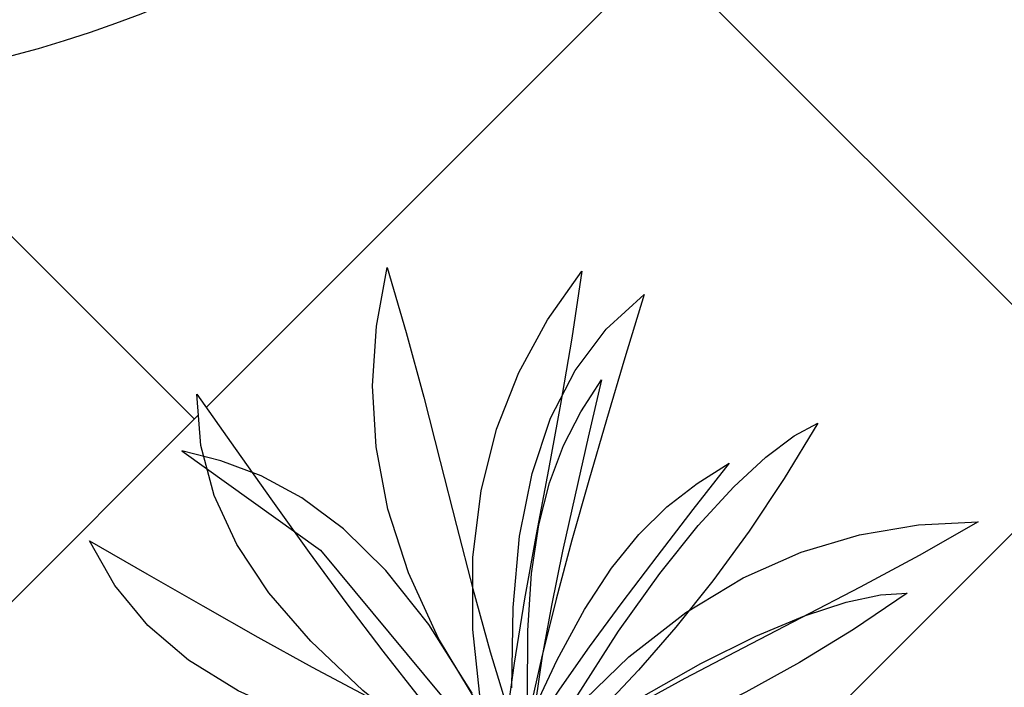
# Model space of a CAD drawing. Units: inches. Extents: x 3590 to 5167, y 65 to 1917.
# Tile 66 of 100: x 4937 to 4968, y 1702 to 1722. Entities that reach past the tile are written whole.
import ezdxf

# ---------------------------------------------------------------- set-up
doc = ezdxf.new("R2010")
doc.units = ezdxf.units.IN
for name, color, linetype, lineweight in [('A-DOOR', 3, 'Continuous', 25), ('A-FLOR-PATT', 8, 'Continuous', 13), ('L-PLNT', 94, 'Continuous', 18)]:
    doc.layers.add(name, color=color, linetype=linetype, lineweight=lineweight)
doc.layers.add('DIENHOA', color=3, linetype='Continuous')

# ---------------------------------------------------------------- blocks, each defined once
blk = doc.blocks.new('Cay03_mb')
at = {"layer": 'DIENHOA'}
for p, q in [((118.6, 555.3), (166.2, 599.1)), ((166.2, 599.1), (142.2, 519.4)), ((79.5, 503.7), (118.6, 555.3)), ((142.2, 519.4), (119, 441.7)), ((48.6, 443.6), (79.5, 503.7)), ((25.5, 374.3), (48.6, 443.6)), ((119, 441.7), (96.7, 365.6)), ((-365.2, 390.3), (-414.4, 402.8)), ((-414.4, 402.8), (-240.2, 277.8)), ((-314.9, 371.3), (-365.2, 390.3)), ((-263.5, 343.5), (-314.9, 371.3)), ((9.9, 295.3), (25.5, 374.3)), ((96.7, 365.6), (75.6, 290.6)), ((-211.2, 304.6), (-263.5, 343.5)), ((436.8, 297.2), (511, 309.6)), ((511, 309.6), (585.9, 313.5)), ((585.9, 313.5), (511.8, 271.4)), ((-158, 252.3), (-211.2, 304.6)), ((363.4, 275.4), (436.8, 297.2)), ((1.6, 205.7), (9.9, 295.3)), ((75.6, 290.6), (55.7, 216.3)), ((-240.2, 277.8), (-88.4, 94.9)), ((290.6, 243.2), (363.4, 275.4)), ((511.8, 271.4), (437.6, 231.5)), ((-104.2, 184.4), (-158, 252.3)), ((218.5, 199.8), (290.6, 243.2)), ((437.6, 231.5), (363.7, 192.9)), ((55.7, 216.3), (37.3, 142.1)), ((0.2, 104.9), (1.6, 205.7)), ((147, 144.1), (218.5, 199.8)), ((363.7, 192.9), (290.2, 154.9)), ((-49.6, 98.5), (-104.2, 184.4)), ((290.2, 154.9), (217.4, 116.6)), ((37.3, 142.1), (20.5, 67.6)), ((75.9, 75.2), (147, 144.1)), ((217.4, 116.6), (145.5, 77.3))]:
    blk.add_line(p, q, dxfattribs=at)
for points in [[(23.7, -5.4), (-41, 82.2), (-91.8, 167.1), (-129.7, 249.5), (-155.6, 329.6), (-170.2, 407.8), (-174.7, 484.2), (-169.8, 559.3), (-156.5, 633.1)], [(-156.5, 633.1), (-132.5, 551.3), (-110.5, 470), (-89.8, 389.2), (-69.6, 309), (-49, 229.4), (-27.1, 150.4), (-3.2, 72.1), (23.7, -5.4)], [(-16.4, -26.7), (-38.3, 80), (-48.9, 178.3), (-48.7, 269), (-38.5, 352.6), (-19.1, 429.7), (9, 501), (44.9, 567.1), (87.9, 628.5)], [(87.9, 628.5), (75.5, 544.2), (61.3, 461.2), (46.1, 379.1), (30.8, 297.8), (16.1, 216.9), (2.9, 136), (-8.3, 54.9), (-16.4, -26.7)], [(23.7, -5.4), (19.8, 93), (20.3, 177), (25, 248.5), (34, 309.8), (47.3, 362.7), (64.9, 409.3), (86.8, 451.7), (112.9, 491.9)], [(112.9, 491.9), (96, 419.7), (79.5, 347.4), (63.9, 276.5), (50, 208.4), (38.4, 144.8), (29.7, 86.9), (24.6, 36.3), (23.7, -5.4)], [(-395.6, 473.7), (-347.5, 405.6), (-300.6, 339.5), (-254.3, 275.1), (-208.3, 212.3), (-161.9, 150.9), (-114.8, 90.7), (-66.5, 31.6), (-16.4, -26.7)], [(-16.4, -26.7), (-108.3, 38.6), (-186.9, 101.7), (-252.4, 163.5), (-305.1, 224.4), (-345.4, 285.2), (-373.7, 346.6), (-390.4, 409.2), (-395.6, 473.7)], [(384.3, 437.5), (342.2, 367.8), (298.1, 301.7), (252.6, 239.4), (206.1, 181.1), (159.4, 127.2), (113, 78), (67.6, 33.6), (23.7, -5.4)], [(23.7, -5.4), (79.9, 91.7), (134.1, 176.2), (185.8, 248.4), (234.3, 308.7), (279, 357.3), (319.3, 394.8), (354.6, 421.4), (384.3, 437.5)], [(273.2, 387.3), (227.6, 328.8), (182.3, 270.1), (138.4, 212.3), (97.2, 156.4), (60, 103.4), (27.8, 54.6), (1.9, 10.8), (-16.4, -26.7)], [(-16.4, -26.7), (21.4, 64.2), (57, 140.3), (91.4, 203.3), (125.2, 255.1), (159.5, 297.5), (195, 332.5), (232.7, 361.8), (273.2, 387.3)], [(-530.5, 289.7), (-458.3, 248.1), (-387.9, 207.8), (-318.9, 168.7), (-250.8, 131.1), (-182.9, 94.8), (-114.9, 59.9), (-46.2, 26.5), (23.7, -5.4)], [(23.7, -5.4), (-87.2, 15.2), (-185, 39.6), (-270.3, 68.2), (-343.7, 101.4), (-405.9, 139.7), (-457.3, 183.5), (-498.7, 233.4), (-530.5, 289.7)], [(496.7, 224), (429.4, 178.4), (361.6, 136.9), (294.1, 99.5), (227.5, 66.1), (162.4, 36.7), (99.7, 11.5), (39.8, -9.7), (-16.4, -26.7)], [(-16.4, -26.7), (75.4, 37.9), (160.1, 91.8), (237.3, 135.7), (306.6, 170), (367.6, 195.4), (419.9, 212.5), (463.1, 221.9), (496.7, 224)]]:
    blk.add_lwpolyline(points, dxfattribs=at)
blk = doc.blocks.new('D1')
at = {"ltscale": 0.5}
blk.add_arc((1, 0), 34, 0, 90, dxfattribs=at)

msp = doc.modelspace()

# ---------------------------------------------------------------- hatches: boundary and pattern name
at = {"layer": 'A-FLOR-PATT', "transparency": 33554687}
h = msp.add_hatch(dxfattribs=at)
h.set_pattern_fill('AR-HBONE', color=256, scale=0.2)
h.set_pattern_definition([(45, (-588.972, 0), (0, 28.73682), [60.96, -20.32]), (135, (-574.604, 14.368), (3e-15, 28.73682), [60.96, -20.32])])
h.paths.add_polyline_path([(5071.274, 1796.999), (4933.274, 1796.999), (4933.274, 1753.999), (4962.774, 1753.999, -0.414214), (4928.774, 1719.999), (4933.274, 1718.999), (4933.274, 1334.999), (5071.274, 1334.999)])
h.paths.add_polyline_path([(4951.78, 1521.077), (4951.715, 1521.04), (4951.563, 1520.895)], flags=16)
h.paths.add_polyline_path([(4952.267, 1521.376), (4952.198, 1521.371), (4952.198, 1521.356)], flags=0)
h.paths.add_polyline_path([(4967.051, 1529.728), (4965.231, 1528.694), (4963.411, 1527.714), (4961.756, 1526.851), (4963.589, 1527.449), (4964.036, 1527.478), (4962.975, 1527.249), (4961.76, 1526.852), (4959.792, 1525.834), (4958.005, 1524.895), (4956.24, 1523.93), (4954.504, 1522.919), (4954.129, 1522.682), (4953.361, 1521.997), (4953.366, 1521.998), (4953.605, 1522.064), (4955.106, 1522.761), (4956.921, 1523.434), (4958.678, 1523.915), (4960.358, 1524.2), (4961.945, 1524.286), (4964.171, 1524.108), (4965.958, 1523.309), (4963.863, 1522.976), (4965.187, 1522.499), (4963.366, 1522.497), (4961.545, 1522.487), (4959.764, 1522.461), (4958.304, 1522.419), (4957.974, 1522.388), (4956.307, 1522.232), (4954.718, 1522.071), (4953.251, 1521.899), (4953.525, 1521.623), (4954.331, 1521.379), (4956.243, 1521.23), (4958.039, 1520.93), (4959.684, 1520.483), (4961.16, 1519.896), (4963.107, 1518.8), (4964.393, 1517.325), (4962.973, 1517.726), (4964.558, 1516.661), (4965.407, 1515.708), (4963.507, 1516.322), (4961.68, 1517.005), (4959.935, 1517.745), (4958.282, 1518.528), (4956.732, 1519.343), (4955.295, 1520.175), (4954.672, 1520.572), (4954.513, 1520.627), (4955.658, 1519.318), (4956.703, 1517.982), (4957.644, 1516.647), (4958.485, 1515.334), (4959.55, 1513.524), (4960.438, 1511.769), (4958.841, 1513.62), (4957.452, 1515.325), (4955.819, 1517.459), (4956.665, 1515.448), (4957.111, 1513.923), (4957.447, 1511.714), (4957.076, 1509.793), (4956.538, 1511.11), (4955.992, 1512.569), (4955.444, 1514.125), (4954.898, 1515.735), (4954.357, 1517.356), (4953.824, 1518.943), (4953.305, 1520.452), (4953.065, 1521.116), (4952.971, 1521.146), (4952.949, 1521.086), (4952.73, 1520.199), (4953.37, 1518.024), (4953.757, 1516.373), (4954.051, 1514.765), (4954.264, 1513.221), (4954.471, 1511.131), (4954.497, 1510.402), (4954.409, 1511.76), (4954.264, 1513.221), (4954.051, 1514.765), (4953.757, 1516.373), (4953.37, 1518.024), (4952.877, 1519.698), (4952.716, 1520.141), (4952.533, 1519.059), (4952.374, 1517.789), (4952.219, 1516.312), (4952.046, 1514.6), (4951.833, 1512.626), (4951.557, 1510.363), (4951.203, 1512.168), (4950.852, 1514.339), (4950.985, 1516.376), (4951.66, 1518.286), (4952.593, 1520.481), (4952.357, 1521.13), (4951.855, 1520.328), (4950.839, 1518.908), (4949.777, 1517.587), (4948.916, 1516.617), (4948.111, 1515.256), (4947.089, 1513.554), (4945.889, 1511.615), (4946.326, 1513.402), (4946.562, 1514.249), (4945.528, 1513.327), (4944.581, 1512.531), (4946.018, 1514.508), (4947.204, 1516.048), (4947.893, 1517.313), (4949.307, 1518.764), (4950.414, 1519.767), (4950.451, 1519.806), (4952.267, 1521.376), (4951.645, 1521.493), (4950.404, 1521.18), (4948.044, 1520.359), (4946.119, 1519.452), (4944.572, 1518.475), (4943.35, 1517.443), (4941.997, 1515.92), (4941.661, 1515.275), (4942.813, 1516.99), (4944.572, 1518.475), (4946.119, 1519.452), (4948.044, 1520.359), (4950.404, 1521.18), (4951.645, 1521.493), (4949.647, 1521.868), (4948.6, 1521.756), (4947.126, 1521.57), (4945.42, 1521.348), (4943.45, 1521.105), (4941.183, 1520.856), (4942.86, 1521.613), (4943.873, 1522.03), (4942.952, 1521.909), (4941.41, 1521.485), (4939.543, 1520.67), (4938.968, 1520.226), (4940.733, 1521.299), (4942.952, 1521.909), (4943.702, 1522.008), (4945.894, 1522.7), (4947.565, 1522.714), (4948.921, 1522.566), (4951.131, 1522.183), (4950.971, 1522.297), (4948.129, 1523.006), (4946.035, 1523.707), (4944.232, 1524.521), (4942.707, 1525.461), (4941.444, 1526.537), (4940.43, 1527.761), (4939.649, 1529.143), (4941.421, 1528.122), (4943.147, 1527.132), (4944.841, 1526.175), (4946.514, 1525.25), (4948.179, 1524.359), (4948.365, 1524.263), (4946.475, 1526.045), (4945.181, 1527.54), (4944.19, 1529.033), (4943.496, 1530.54), (4943.278, 1531.36), (4942.498, 1531.919), (4943.114, 1531.762), (4942.959, 1533.659), (4944.14, 1531.989), (4944.612, 1531.323), (4946.202, 1530.463), (4947.486, 1529.509), (4948.79, 1528.226), (4950.368, 1526.237), (4949.485, 1528.155), (4948.851, 1530.123), (4948.491, 1532.041), (4948.381, 1533.918), (4948.501, 1535.76), (4948.827, 1537.573), (4949.418, 1535.565), (4949.957, 1533.569), (4950.464, 1531.586), (4950.961, 1529.617), (4951.391, 1527.954), (4951.724, 1530.687), (4952.201, 1532.58), (4952.889, 1534.33), (4953.77, 1535.951), (4954.827, 1537.46), (4954.521, 1535.39), (4954.273, 1533.937), (4955.58, 1535.663), (4956.748, 1536.739), (4956.159, 1534.78), (4955.589, 1532.873), (4955.043, 1531.006), (4954.525, 1529.166), (4954.038, 1527.341), (4953.638, 1525.733), (4953.611, 1525.586), (4953.398, 1524.166), (4953.382, 1524.009), (4954.07, 1525.476), (4954.912, 1527.022), (4956.136, 1528.894), (4957.847, 1530.577), (4959.376, 1531.54), (4958.256, 1530.104), (4957.143, 1528.663), (4956.066, 1527.243), (4955.056, 1525.871), (4954.141, 1524.571), (4953.352, 1523.372), (4953.311, 1523.303), (4953.273, 1522.925), (4953.261, 1522.382), (4954.103, 1523.373), (4954.63, 1524.284), (4955.961, 1526.358), (4957.23, 1528.13), (4958.421, 1529.609), (4960.037, 1531.368), (4961.374, 1532.375), (4962.101, 1532.77), (4961.07, 1531.061), (4959.987, 1529.438), (4958.869, 1527.908), (4958.15, 1527.007), (4959.803, 1528.003), (4961.589, 1528.793), (4963.391, 1529.328), (4965.211, 1529.632)], flags=16)
h.paths.add_polyline_path([(4962.944, 1523.182), (4961.107, 1523.422), (4960.392, 1523.362), (4962.35, 1523.331)], flags=0)
h.paths.add_polyline_path([(5049.541, 1584.551), (5049.476, 1584.515), (5049.325, 1584.37)], flags=16)
h.paths.add_polyline_path([(5050.028, 1584.851), (5049.959, 1584.845), (5049.959, 1584.83)], flags=0)
h.paths.add_polyline_path([(5042.333, 1581.949), (5043.88, 1582.926), (5045.806, 1583.833), (5048.165, 1584.654), (5049.406, 1584.967), (5047.408, 1585.342), (5046.361, 1585.231), (5044.888, 1585.044), (5043.181, 1584.822), (5041.211, 1584.579), (5038.944, 1584.33), (5040.622, 1585.087), (5041.634, 1585.504), (5040.713, 1585.383), (5039.171, 1584.959), (5037.304, 1584.144), (5036.729, 1583.7), (5038.494, 1584.773), (5040.713, 1585.383), (5041.463, 1585.482), (5043.655, 1586.174), (5045.326, 1586.188), (5046.682, 1586.04), (5048.893, 1585.657), (5048.732, 1585.771), (5045.891, 1586.48), (5043.796, 1587.181), (5041.994, 1587.996), (5040.468, 1588.935), (5039.205, 1590.011), (5038.191, 1591.235), (5037.41, 1592.617), (5039.182, 1591.596), (5040.909, 1590.607), (5042.602, 1589.649), (5044.275, 1588.724), (5045.94, 1587.833), (5046.126, 1587.738), (5044.237, 1589.519), (5042.942, 1591.015), (5041.952, 1592.508), (5041.257, 1594.014), (5041.039, 1594.834), (5040.26, 1595.393), (5040.875, 1595.237), (5040.721, 1597.133), (5041.901, 1595.463), (5042.373, 1594.798), (5043.963, 1593.938), (5045.247, 1592.983), (5046.552, 1591.701), (5048.129, 1589.712), (5047.247, 1591.63), (5046.613, 1593.597), (5046.252, 1595.515), (5046.142, 1597.392), (5046.262, 1599.234), (5046.588, 1601.047), (5047.179, 1599.039), (5047.718, 1597.043), (5048.225, 1595.06), (5048.722, 1593.091), (5049.152, 1591.429), (5049.485, 1594.161), (5049.962, 1596.054), (5050.65, 1597.804), (5051.532, 1599.425), (5052.589, 1600.934), (5052.283, 1598.864), (5052.034, 1597.411), (5053.341, 1599.137), (5054.509, 1600.213), (5053.92, 1598.254), (5053.35, 1596.348), (5052.805, 1594.48), (5052.286, 1592.64), (5051.799, 1590.815), (5051.4, 1589.207), (5051.373, 1589.06), (5051.159, 1587.64), (5051.143, 1587.483), (5051.831, 1588.95), (5052.673, 1590.496), (5053.898, 1592.368), (5055.608, 1594.051), (5057.137, 1595.014), (5056.017, 1593.578), (5054.904, 1592.137), (5053.828, 1590.717), (5052.817, 1589.345), (5051.902, 1588.046), (5051.113, 1586.846), (5051.072, 1586.777), (5051.034, 1586.399), (5051.022, 1585.856), (5051.864, 1586.847), (5052.391, 1587.758), (5053.723, 1589.832), (5054.991, 1591.604), (5056.182, 1593.083), (5057.798, 1594.842), (5059.135, 1595.849), (5059.863, 1596.244), (5058.831, 1594.535), (5057.749, 1592.912), (5056.63, 1591.382), (5055.912, 1590.482), (5057.564, 1591.477), (5059.35, 1592.267), (5061.152, 1592.802), (5062.972, 1593.106), (5064.812, 1593.203), (5062.992, 1592.169), (5061.172, 1591.188), (5059.518, 1590.325), (5061.35, 1590.924), (5061.797, 1590.952), (5060.737, 1590.723), (5059.521, 1590.326), (5057.553, 1589.308), (5055.766, 1588.369), (5054.002, 1587.404), (5052.265, 1586.393), (5051.891, 1586.156), (5051.122, 1585.471), (5051.127, 1585.472), (5051.366, 1585.538), (5052.867, 1586.235), (5054.682, 1586.908), (5056.439, 1587.389), (5058.12, 1587.675), (5059.706, 1587.76), (5061.933, 1587.583), (5063.719, 1586.783), (5061.624, 1586.45), (5062.949, 1585.973), (5061.127, 1585.971), (5059.307, 1585.961), (5057.525, 1585.935), (5056.065, 1585.893), (5055.735, 1585.862), (5054.068, 1585.707), (5052.479, 1585.546), (5051.012, 1585.373), (5051.286, 1585.097), (5052.092, 1584.853), (5054.004, 1584.704), (5055.8, 1584.404), (5057.446, 1583.958), (5058.921, 1583.37), (5060.868, 1582.274), (5062.154, 1580.799), (5060.734, 1581.2), (5062.32, 1580.135), (5063.168, 1579.182), (5061.269, 1579.796), (5059.441, 1580.479), (5057.696, 1581.219), (5056.043, 1582.003), (5054.493, 1582.817), (5053.057, 1583.649), (5052.433, 1584.047), (5052.274, 1584.101), (5053.42, 1582.793), (5054.464, 1581.457), (5055.405, 1580.121), (5056.247, 1578.809), (5057.311, 1576.998), (5058.199, 1575.244), (5056.602, 1577.094), (5055.213, 1578.799), (5053.58, 1580.933), (5054.427, 1578.922), (5054.872, 1577.397), (5055.208, 1575.189), (5054.838, 1573.267), (5054.299, 1574.584), (5053.754, 1576.043), (5053.206, 1577.599), (5052.659, 1579.209), (5052.118, 1580.83), (5051.585, 1582.417), (5051.066, 1583.927), (5050.826, 1584.59), (5050.733, 1584.62), (5050.711, 1584.561), (5050.491, 1583.673), (5051.131, 1581.498), (5051.518, 1579.847), (5051.813, 1578.24), (5052.026, 1576.695), (5052.233, 1574.605), (5052.258, 1573.876), (5052.17, 1575.234), (5052.026, 1576.695), (5051.813, 1578.24), (5051.518, 1579.847), (5051.131, 1581.498), (5050.638, 1583.172), (5050.477, 1583.615), (5050.294, 1582.533), (5050.136, 1581.263), (5049.981, 1579.786), (5049.807, 1578.074), (5049.594, 1576.1), (5049.318, 1573.837), (5048.965, 1575.642), (5048.613, 1577.813), (5048.747, 1579.85), (5049.421, 1581.76), (5050.354, 1583.955), (5050.118, 1584.604), (5049.616, 1583.802), (5048.6, 1582.382), (5047.538, 1581.061), (5046.677, 1580.091), (5045.872, 1578.73), (5044.85, 1577.028), (5043.651, 1575.089), (5044.087, 1576.877), (5044.324, 1577.723), (5043.289, 1576.801), (5042.342, 1576.005), (5043.779, 1577.982), (5044.966, 1579.522), (5045.655, 1580.787), (5047.068, 1582.239), (5048.175, 1583.241), (5048.213, 1583.28), (5050.028, 1584.851), (5049.406, 1584.967), (5048.165, 1584.654), (5045.806, 1583.833), (5043.88, 1582.926), (5042.333, 1581.949), (5041.111, 1580.917), (5039.758, 1579.394), (5039.423, 1578.749), (5040.575, 1580.464)], flags=16)
h.paths.add_polyline_path([(4954.799, 1533.12), (4954.262, 1532.079), (4953.831, 1530.935), (4953.505, 1529.636), (4953.283, 1528.133), (4953.167, 1526.376), (4953.156, 1524.315), (4953.277, 1521.236), (4952.802, 1521.842), (4951.557, 1521.998), (4950.976, 1521.961), (4952.661, 1521.941), (4952.802, 1521.842), (4953.152, 1523.593), (4953.167, 1526.376), (4953.283, 1528.133), (4953.609, 1530.346), (4954.456, 1532.592)], flags=0)
h.paths.add_polyline_path([(5050.563, 1585.316), (5049.318, 1585.472), (5048.737, 1585.435), (5050.422, 1585.415), (5050.563, 1585.316), (5050.914, 1587.067), (5050.928, 1589.851), (5051.045, 1591.607), (5051.371, 1593.82), (5052.217, 1596.066), (5052.56, 1596.594), (5052.024, 1595.554), (5051.592, 1594.409), (5051.266, 1593.11), (5051.045, 1591.607), (5050.928, 1589.851), (5050.918, 1587.789), (5051.038, 1584.71)], flags=0)
h.paths.add_polyline_path([(5058.153, 1586.836), (5060.111, 1586.805), (5060.705, 1586.656), (5058.868, 1586.896)], flags=0)
h.paths.add_polyline_path([(5049.541, 1430.936), (5049.476, 1430.9), (5049.325, 1430.755)], flags=16)
h.paths.add_polyline_path([(5050.028, 1431.236), (5049.959, 1431.231), (5049.959, 1431.215)], flags=0)
h.paths.add_polyline_path([(5046.588, 1447.432), (5047.179, 1445.425), (5047.718, 1443.429), (5048.225, 1441.446), (5048.722, 1439.476), (5049.152, 1437.814), (5049.485, 1440.546), (5049.962, 1442.439), (5050.65, 1444.189), (5051.532, 1445.811), (5052.589, 1447.319), (5052.283, 1445.249), (5052.034, 1443.796), (5053.341, 1445.522), (5054.509, 1446.598), (5053.92, 1444.64), (5053.35, 1442.733), (5052.805, 1440.865), (5052.286, 1439.025), (5051.799, 1437.201), (5051.4, 1435.592), (5051.373, 1435.445), (5051.159, 1434.025), (5051.143, 1433.868), (5051.831, 1435.335), (5052.673, 1436.881), (5053.898, 1438.753), (5055.608, 1440.436), (5057.137, 1441.4), (5056.017, 1439.963), (5054.904, 1438.522), (5053.828, 1437.102), (5052.817, 1435.73), (5051.902, 1434.431), (5051.113, 1433.231), (5051.072, 1433.162), (5051.034, 1432.784), (5051.022, 1432.242), (5051.864, 1433.232), (5052.391, 1434.143), (5053.723, 1436.217), (5054.991, 1437.989), (5056.182, 1439.468), (5057.798, 1441.227), (5059.135, 1442.235), (5059.863, 1442.629), (5058.831, 1440.921), (5057.749, 1439.298), (5056.63, 1437.767), (5055.912, 1436.867), (5057.564, 1437.863), (5059.35, 1438.652), (5061.152, 1439.187), (5062.972, 1439.491), (5064.812, 1439.588), (5062.992, 1438.554), (5061.172, 1437.573), (5059.518, 1436.71), (5061.35, 1437.309), (5061.797, 1437.337), (5060.737, 1437.108), (5059.521, 1436.711), (5057.553, 1435.693), (5055.766, 1434.754), (5054.002, 1433.789), (5052.265, 1432.778), (5051.891, 1432.541), (5051.122, 1431.856), (5051.127, 1431.857), (5051.366, 1431.923), (5052.867, 1432.62), (5054.682, 1433.293), (5056.439, 1433.775), (5058.12, 1434.06), (5059.706, 1434.145), (5061.933, 1433.968), (5063.719, 1433.168), (5061.624, 1432.835), (5062.949, 1432.358), (5061.127, 1432.357), (5059.307, 1432.346), (5057.525, 1432.32), (5056.065, 1432.278), (5055.735, 1432.248), (5054.068, 1432.092), (5052.479, 1431.931), (5051.012, 1431.759), (5051.286, 1431.482), (5052.092, 1431.238), (5054.004, 1431.089), (5055.8, 1430.789), (5057.446, 1430.343), (5058.921, 1429.755), (5060.868, 1428.66), (5062.154, 1427.185), (5060.734, 1427.585), (5062.32, 1426.52), (5063.168, 1425.567), (5061.269, 1426.181), (5059.441, 1426.865), (5057.696, 1427.604), (5056.043, 1428.388), (5054.493, 1429.202), (5053.057, 1430.034), (5052.433, 1430.432), (5052.274, 1430.487), (5053.42, 1429.178), (5054.464, 1427.842), (5055.405, 1426.506), (5056.247, 1425.194), (5057.311, 1423.383), (5058.199, 1421.629), (5056.602, 1423.479), (5055.213, 1425.184), (5053.58, 1427.318), (5054.427, 1425.307), (5054.872, 1423.782), (5055.208, 1421.574), (5054.838, 1419.652), (5054.299, 1420.97), (5053.754, 1422.428), (5053.206, 1423.984), (5052.659, 1425.595), (5052.118, 1427.215), (5051.585, 1428.802), (5051.066, 1430.312), (5050.826, 1430.975), (5050.733, 1431.005), (5050.711, 1430.946), (5050.491, 1430.058), (5051.131, 1427.883), (5051.518, 1426.232), (5051.813, 1424.625), (5052.026, 1423.081), (5052.233, 1420.991), (5052.258, 1420.261), (5052.17, 1421.619), (5052.026, 1423.081), (5051.813, 1424.625), (5051.518, 1426.232), (5051.131, 1427.883), (5050.638, 1429.558), (5050.477, 1430.001), (5050.294, 1428.918), (5050.136, 1427.648), (5049.981, 1426.171), (5049.807, 1424.459), (5049.594, 1422.485), (5049.318, 1420.222), (5048.965, 1422.028), (5048.613, 1424.199), (5048.747, 1426.235), (5049.421, 1428.146), (5050.354, 1430.34), (5050.118, 1430.989), (5049.616, 1430.187), (5048.6, 1428.768), (5047.538, 1427.446), (5046.677, 1426.477), (5045.872, 1425.116), (5044.85, 1423.413), (5043.651, 1421.474), (5044.087, 1423.262), (5044.324, 1424.109), (5043.289, 1423.186), (5042.342, 1422.391), (5043.779, 1424.368), (5044.966, 1425.907), (5045.655, 1427.173), (5047.068, 1428.624), (5048.175, 1429.627), (5048.213, 1429.666), (5050.028, 1431.236), (5049.406, 1431.353), (5048.165, 1431.039), (5045.806, 1430.218), (5043.88, 1429.311), (5042.333, 1428.334), (5041.111, 1427.302), (5039.758, 1425.779), (5039.423, 1425.134), (5040.575, 1426.849), (5042.333, 1428.334), (5043.88, 1429.311), (5045.806, 1430.218), (5048.165, 1431.039), (5049.406, 1431.353), (5047.408, 1431.727), (5046.361, 1431.616), (5044.888, 1431.429), (5043.181, 1431.207), (5041.211, 1430.964), (5038.944, 1430.715), (5040.622, 1431.472), (5041.634, 1431.89), (5040.713, 1431.769), (5039.171, 1431.345), (5037.304, 1430.53), (5036.729, 1430.085), (5038.494, 1431.158), (5040.713, 1431.769), (5041.463, 1431.867), (5043.655, 1432.559), (5045.326, 1432.573), (5046.682, 1432.425), (5048.893, 1432.042), (5048.732, 1432.156), (5045.891, 1432.865), (5043.796, 1433.566), (5041.994, 1434.381), (5040.468, 1435.321), (5039.205, 1436.396), (5038.191, 1437.62), (5037.41, 1439.002), (5039.182, 1437.982), (5040.909, 1436.992), (5042.602, 1436.034), (5044.275, 1435.109), (5045.94, 1434.218), (5046.126, 1434.123), (5044.237, 1435.904), (5042.942, 1437.4), (5041.952, 1438.893), (5041.257, 1440.399), (5041.039, 1441.219), (5040.26, 1441.778), (5040.875, 1441.622), (5040.721, 1443.518), (5041.901, 1441.848), (5042.373, 1441.183), (5043.963, 1440.323), (5045.247, 1439.369), (5046.552, 1438.086), (5048.129, 1436.097), (5047.247, 1438.015), (5046.613, 1439.982), (5046.252, 1441.901), (5046.142, 1443.778), (5046.262, 1445.619)], flags=16)
h.paths.add_polyline_path([(5052.382, 1444.255), (5051.623, 1442.78), (5052.024, 1441.939), (5052.56, 1442.98)], flags=0)
h.paths.add_polyline_path([(5050.563, 1431.701), (5049.318, 1431.857), (5048.737, 1431.821), (5050.422, 1431.8)], flags=0)
h.paths.add_polyline_path([(5058.153, 1433.221), (5060.111, 1433.19), (5060.705, 1433.041), (5058.868, 1433.281)], flags=0)
h.paths.add_polyline_path([(5049.541, 1352.285), (5049.476, 1352.249), (5049.325, 1352.104)], flags=16)
h.paths.add_polyline_path([(5050.028, 1352.585), (5049.959, 1352.58), (5049.959, 1352.564)], flags=0)
h.paths.add_polyline_path([(5046.588, 1368.781), (5047.179, 1366.774), (5047.718, 1364.778), (5048.225, 1362.795), (5048.722, 1360.825), (5049.152, 1359.163), (5049.485, 1361.896), (5049.962, 1363.789), (5050.65, 1365.538), (5051.532, 1367.16), (5052.589, 1368.669), (5052.283, 1366.598), (5052.034, 1365.145), (5053.341, 1366.871), (5054.509, 1367.947), (5053.92, 1365.989), (5053.35, 1364.082), (5052.805, 1362.214), (5052.286, 1360.374), (5051.799, 1358.55), (5051.4, 1356.942), (5051.373, 1356.794), (5051.159, 1355.374), (5051.143, 1355.218), (5051.831, 1356.684), (5052.673, 1358.23), (5053.898, 1360.102), (5055.608, 1361.786), (5057.137, 1362.749), (5056.017, 1361.313), (5054.904, 1359.872), (5053.828, 1358.452), (5052.817, 1357.079), (5051.902, 1355.78), (5051.113, 1354.581), (5051.072, 1354.512), (5051.034, 1354.133), (5051.022, 1353.591), (5051.864, 1354.581), (5052.391, 1355.492), (5053.723, 1357.566), (5054.991, 1359.338), (5056.182, 1360.817), (5057.798, 1362.577), (5059.135, 1363.584), (5059.863, 1363.979), (5058.831, 1362.27), (5057.749, 1360.647), (5056.63, 1359.117), (5055.912, 1358.216), (5057.564, 1359.212), (5059.35, 1360.001), (5061.152, 1360.536), (5062.972, 1360.841), (5064.812, 1360.937), (5062.992, 1359.903), (5061.172, 1358.923), (5059.518, 1358.059), (5061.35, 1358.658), (5061.797, 1358.687), (5060.737, 1358.458), (5059.521, 1358.061), (5057.553, 1357.043), (5055.766, 1356.103), (5054.002, 1355.138), (5052.265, 1354.127), (5051.891, 1353.89), (5051.122, 1353.206), (5051.127, 1353.206), (5051.366, 1353.272), (5052.867, 1353.969), (5054.682, 1354.643), (5056.439, 1355.124), (5058.12, 1355.409), (5059.706, 1355.495), (5061.933, 1355.317), (5063.719, 1354.518), (5061.624, 1354.184), (5062.949, 1353.708), (5061.127, 1353.706), (5059.307, 1353.695), (5057.525, 1353.669), (5056.065, 1353.627), (5055.735, 1353.597), (5054.068, 1353.441), (5052.479, 1353.28), (5051.012, 1353.108), (5051.286, 1352.831), (5052.092, 1352.587), (5054.004, 1352.439), (5055.8, 1352.138), (5057.446, 1351.692), (5058.921, 1351.104), (5060.868, 1350.009), (5062.154, 1348.534), (5060.734, 1348.935), (5062.32, 1347.869), (5063.168, 1346.916), (5061.269, 1347.53), (5059.441, 1348.214), (5057.696, 1348.954), (5056.043, 1349.737), (5054.493, 1350.551), (5053.057, 1351.383), (5052.433, 1351.781), (5052.274, 1351.836), (5053.42, 1350.527), (5054.464, 1349.191), (5055.405, 1347.855), (5056.247, 1346.543), (5057.311, 1344.733), (5058.199, 1342.978), (5056.602, 1344.828), (5055.213, 1346.534), (5053.58, 1348.667), (5054.427, 1346.656), (5054.872, 1345.132), (5055.208, 1342.923), (5054.838, 1341.002), (5054.299, 1342.319), (5053.754, 1343.778), (5053.206, 1345.334), (5052.659, 1346.944), (5052.118, 1348.564), (5051.585, 1350.151), (5051.066, 1351.661), (5050.826, 1352.324), (5050.733, 1352.355), (5050.711, 1352.295), (5050.491, 1351.408), (5051.131, 1349.232), (5051.518, 1347.581), (5051.813, 1345.974), (5052.026, 1344.43), (5052.233, 1342.34), (5052.258, 1341.61), (5052.17, 1342.969), (5052.026, 1344.43), (5051.813, 1345.974), (5051.518, 1347.581), (5051.131, 1349.232), (5050.638, 1350.907), (5050.477, 1351.35), (5050.294, 1350.267), (5050.136, 1348.997), (5049.981, 1347.52), (5049.807, 1345.809), (5049.594, 1343.835), (5049.318, 1341.571), (5048.965, 1343.377), (5048.613, 1345.548), (5048.747, 1347.585), (5049.421, 1349.495), (5050.354, 1351.689), (5050.118, 1352.339), (5049.616, 1351.536), (5048.6, 1350.117), (5047.538, 1348.795), (5046.677, 1347.826), (5045.872, 1346.465), (5044.85, 1344.763), (5043.651, 1342.824), (5044.087, 1344.611), (5044.324, 1345.458), (5043.289, 1344.535), (5042.342, 1343.74), (5043.779, 1345.717), (5044.966, 1347.256), (5045.655, 1348.522), (5047.068, 1349.973), (5048.175, 1350.976), (5048.213, 1351.015), (5050.028, 1352.585), (5049.406, 1352.702), (5048.165, 1352.388), (5045.806, 1351.567), (5043.88, 1350.661), (5042.333, 1349.683), (5041.111, 1348.651), (5039.758, 1347.128), (5039.423, 1346.483), (5040.575, 1348.198), (5042.333, 1349.683), (5043.88, 1350.661), (5045.806, 1351.567), (5048.165, 1352.388), (5049.406, 1352.702), (5047.408, 1353.076), (5046.361, 1352.965), (5044.888, 1352.779), (5043.181, 1352.556), (5041.211, 1352.313), (5038.944, 1352.065), (5040.622, 1352.821), (5041.634, 1353.239), (5040.713, 1353.118), (5039.171, 1352.694), (5037.304, 1351.879), (5036.729, 1351.434), (5038.494, 1352.508), (5040.713, 1353.118), (5041.463, 1353.216), (5043.655, 1353.909), (5045.326, 1353.923), (5046.682, 1353.774), (5048.893, 1353.391), (5048.732, 1353.506), (5045.891, 1354.214), (5043.796, 1354.915), (5041.994, 1355.73), (5040.468, 1356.67), (5039.205, 1357.746), (5038.191, 1358.969), (5037.41, 1360.352), (5039.182, 1359.331), (5040.909, 1358.341), (5042.602, 1357.383), (5044.275, 1356.458), (5045.94, 1355.567), (5046.126, 1355.472), (5044.237, 1357.253), (5042.942, 1358.749), (5041.952, 1360.242), (5041.257, 1361.748), (5041.039, 1362.568), (5040.26, 1363.128), (5040.875, 1362.971), (5040.721, 1364.867), (5041.901, 1363.197), (5042.373, 1362.532), (5043.963, 1361.672), (5045.247, 1360.718), (5046.552, 1359.435), (5048.129, 1357.446), (5047.247, 1359.364), (5046.613, 1361.331), (5046.252, 1363.25), (5046.142, 1365.127), (5046.262, 1366.969)], flags=16)
h.paths.add_polyline_path([(5052.382, 1365.604), (5051.623, 1364.129), (5052.024, 1363.288), (5052.56, 1364.329)], flags=0)
h.paths.add_polyline_path([(4951.78, 1698.041), (4951.715, 1698.005), (4951.563, 1697.859)], flags=16)
h.paths.add_polyline_path([(4952.267, 1698.341), (4952.198, 1698.335), (4952.198, 1698.32)], flags=0)
h.paths.add_polyline_path([(4957.076, 1686.757), (4956.538, 1688.074), (4955.992, 1689.533), (4955.444, 1691.089), (4954.898, 1692.699), (4954.357, 1694.32), (4953.824, 1695.907), (4953.305, 1697.417), (4953.065, 1698.08), (4952.971, 1698.11), (4952.949, 1698.051), (4952.73, 1697.163), (4953.37, 1694.988), (4953.757, 1693.337), (4954.051, 1691.729), (4954.264, 1690.185), (4954.471, 1688.095), (4954.497, 1687.366), (4954.409, 1688.724), (4954.264, 1690.185), (4954.051, 1691.729), (4953.757, 1693.337), (4953.37, 1694.988), (4952.877, 1696.662), (4952.716, 1697.105), (4952.533, 1696.023), (4952.374, 1694.753), (4952.219, 1693.276), (4952.046, 1691.564), (4951.833, 1689.59), (4951.557, 1687.327), (4951.203, 1689.132), (4950.852, 1691.303), (4950.985, 1693.34), (4951.66, 1695.25), (4952.593, 1697.445), (4952.357, 1698.094), (4951.855, 1697.292), (4950.839, 1695.872), (4949.777, 1694.551), (4948.916, 1693.581), (4948.111, 1692.22), (4947.089, 1690.518), (4945.889, 1688.579), (4946.326, 1690.366), (4946.562, 1691.213), (4945.528, 1690.291), (4944.581, 1689.495), (4946.018, 1691.472), (4947.204, 1693.012), (4947.893, 1694.277), (4949.307, 1695.729), (4950.414, 1696.731), (4950.451, 1696.77), (4952.267, 1698.341), (4951.645, 1698.457), (4950.404, 1698.144), (4948.044, 1697.323), (4946.119, 1696.416), (4944.572, 1695.439), (4943.35, 1694.407), (4941.997, 1692.884), (4941.661, 1692.239), (4942.813, 1693.954), (4944.572, 1695.439), (4946.119, 1696.416), (4948.044, 1697.323), (4950.404, 1698.144), (4951.645, 1698.457), (4949.647, 1698.832), (4948.6, 1698.72), (4947.126, 1698.534), (4945.42, 1698.312), (4943.45, 1698.069), (4941.183, 1697.82), (4942.86, 1698.577), (4943.873, 1698.994), (4942.952, 1698.873), (4941.41, 1698.449), (4939.543, 1697.634), (4938.968, 1697.19), (4940.733, 1698.263), (4942.952, 1698.873), (4943.702, 1698.972), (4945.894, 1699.664), (4947.565, 1699.678), (4948.921, 1699.53), (4951.131, 1699.147), (4950.971, 1699.261), (4948.129, 1699.97), (4946.035, 1700.671), (4944.232, 1701.486), (4942.707, 1702.425), (4941.444, 1703.501), (4940.43, 1704.725), (4939.649, 1706.107), (4941.421, 1705.086), (4943.147, 1704.097), (4944.841, 1703.139), (4946.514, 1702.214), (4948.179, 1701.323), (4948.365, 1701.227), (4946.475, 1703.009), (4945.181, 1704.505), (4944.19, 1705.997), (4943.496, 1707.504), (4943.278, 1708.324), (4942.498, 1708.883), (4943.114, 1708.727), (4942.959, 1710.623), (4944.14, 1708.953), (4944.612, 1708.287), (4946.202, 1707.428), (4947.486, 1706.473), (4948.79, 1705.191), (4950.368, 1703.202), (4949.485, 1705.12), (4948.851, 1707.087), (4948.491, 1709.005), (4948.381, 1710.882), (4948.501, 1712.724), (4948.827, 1714.537), (4949.418, 1712.529), (4949.957, 1710.533), (4950.464, 1708.55), (4950.961, 1706.581), (4951.391, 1704.919), (4951.724, 1707.651), (4952.201, 1709.544), (4952.889, 1711.294), (4953.77, 1712.915), (4954.827, 1714.424), (4954.521, 1712.354), (4954.273, 1710.901), (4955.58, 1712.627), (4956.748, 1713.703), (4956.159, 1711.744), (4955.589, 1709.837), (4955.043, 1707.97), (4954.525, 1706.13), (4954.038, 1704.305), (4953.638, 1702.697), (4953.611, 1702.55), (4953.398, 1701.13), (4953.382, 1700.973), (4954.07, 1702.44), (4954.912, 1703.986), (4956.136, 1705.858), (4957.847, 1707.541), (4959.376, 1708.504), (4958.256, 1707.068), (4957.143, 1705.627), (4956.066, 1704.207), (4955.056, 1702.835), (4954.141, 1701.536), (4953.352, 1700.336), (4953.311, 1700.267), (4953.273, 1699.889), (4953.261, 1699.346), (4954.103, 1700.337), (4954.63, 1701.248), (4955.961, 1703.322), (4957.23, 1705.094), (4958.421, 1706.573), (4960.037, 1708.332), (4961.374, 1709.339), (4962.101, 1709.734), (4961.07, 1708.025), (4959.987, 1706.402), (4958.869, 1704.872), (4958.15, 1703.972), (4959.803, 1704.967), (4961.589, 1705.757), (4963.391, 1706.292), (4965.211, 1706.596), (4967.051, 1706.692), (4965.231, 1705.659), (4963.411, 1704.678), (4961.756, 1703.815), (4963.589, 1704.413), (4964.036, 1704.442), (4962.975, 1704.213), (4961.76, 1703.816), (4959.792, 1702.798), (4958.005, 1701.859), (4956.24, 1700.894), (4954.504, 1699.883), (4954.129, 1699.646), (4953.361, 1698.961), (4953.366, 1698.962), (4953.605, 1699.028), (4955.106, 1699.725), (4956.921, 1700.398), (4958.678, 1700.879), (4960.358, 1701.164), (4961.945, 1701.25), (4964.171, 1701.073), (4965.958, 1700.273), (4963.863, 1699.94), (4965.187, 1699.463), (4963.366, 1699.461), (4961.545, 1699.451), (4959.764, 1699.425), (4958.304, 1699.383), (4957.974, 1699.352), (4956.307, 1699.197), (4954.718, 1699.036), (4953.251, 1698.863), (4953.525, 1698.587), (4954.331, 1698.343), (4956.243, 1698.194), (4958.039, 1697.894), (4959.684, 1697.447), (4961.16, 1696.86), (4963.107, 1695.764), (4964.393, 1694.289), (4962.973, 1694.69), (4964.558, 1693.625), (4965.407, 1692.672), (4963.507, 1693.286), (4961.68, 1693.969), (4959.935, 1694.709), (4958.282, 1695.492), (4956.732, 1696.307), (4955.295, 1697.139), (4954.672, 1697.536), (4954.513, 1697.591), (4955.658, 1696.282), (4956.703, 1694.946), (4957.644, 1693.611), (4958.485, 1692.298), (4959.55, 1690.488), (4960.438, 1688.733), (4958.841, 1690.584), (4957.452, 1692.289), (4955.819, 1694.423), (4956.665, 1692.412), (4957.111, 1690.887), (4957.447, 1688.678)], flags=16)
h.paths.add_polyline_path([(5050.563, 1353.05), (5049.318, 1353.207), (5048.737, 1353.17), (5050.422, 1353.15)], flags=0)
h.paths.add_polyline_path([(4951.78, 1351.486), (4951.715, 1351.45), (4951.563, 1351.305)], flags=16)
h.paths.add_polyline_path([(4952.267, 1351.786), (4952.198, 1351.78), (4952.198, 1351.765)], flags=0)
h.paths.add_polyline_path([(4954.827, 1367.869), (4954.521, 1365.799), (4954.273, 1364.346), (4955.58, 1366.072), (4956.748, 1367.148), (4956.159, 1365.19), (4955.589, 1363.283), (4955.043, 1361.415), (4954.525, 1359.575), (4954.038, 1357.751), (4953.638, 1356.142), (4953.611, 1355.995), (4953.398, 1354.575), (4953.382, 1354.418), (4954.07, 1355.885), (4954.912, 1357.431), (4956.136, 1359.303), (4957.847, 1360.986), (4959.376, 1361.95), (4958.256, 1360.513), (4957.143, 1359.072), (4956.066, 1357.652), (4955.056, 1356.28), (4954.141, 1354.981), (4953.352, 1353.781), (4953.311, 1353.712), (4953.273, 1353.334), (4953.261, 1352.792), (4954.103, 1353.782), (4954.63, 1354.693), (4955.961, 1356.767), (4957.23, 1358.539), (4958.421, 1360.018), (4960.037, 1361.777), (4961.374, 1362.785), (4962.101, 1363.179), (4961.07, 1361.471), (4959.987, 1359.848), (4958.869, 1358.317), (4958.15, 1357.417), (4959.803, 1358.413), (4961.589, 1359.202), (4963.391, 1359.737), (4965.211, 1360.041), (4967.051, 1360.138), (4965.231, 1359.104), (4963.411, 1358.123), (4961.756, 1357.26), (4963.589, 1357.859), (4964.036, 1357.887), (4962.975, 1357.658), (4961.76, 1357.261), (4959.792, 1356.243), (4958.005, 1355.304), (4956.24, 1354.339), (4954.504, 1353.328), (4954.129, 1353.091), (4953.361, 1352.406), (4953.366, 1352.407), (4953.605, 1352.473), (4955.106, 1353.17), (4956.921, 1353.843), (4958.678, 1354.325), (4960.358, 1354.61), (4961.945, 1354.695), (4964.171, 1354.518), (4965.958, 1353.718), (4963.863, 1353.385), (4965.187, 1352.908), (4963.366, 1352.907), (4961.545, 1352.896), (4959.764, 1352.87), (4958.304, 1352.828), (4957.974, 1352.798), (4956.307, 1352.642), (4954.718, 1352.481), (4953.251, 1352.309), (4953.525, 1352.032), (4954.331, 1351.788), (4956.243, 1351.639), (4958.039, 1351.339), (4959.684, 1350.893), (4961.16, 1350.305), (4963.107, 1349.21), (4964.393, 1347.735), (4962.973, 1348.135), (4964.558, 1347.07), (4965.407, 1346.117), (4963.507, 1346.731), (4961.68, 1347.414), (4959.935, 1348.154), (4958.282, 1348.938), (4956.732, 1349.752), (4955.295, 1350.584), (4954.672, 1350.982), (4954.513, 1351.036), (4955.658, 1349.728), (4956.703, 1348.392), (4957.644, 1347.056), (4958.485, 1345.744), (4959.55, 1343.933), (4960.438, 1342.179), (4958.841, 1344.029), (4957.452, 1345.734), (4955.819, 1347.868), (4956.665, 1345.857), (4957.111, 1344.332), (4957.447, 1342.124), (4957.076, 1340.202), (4956.538, 1341.52), (4955.992, 1342.978), (4955.444, 1344.534), (4954.898, 1346.145), (4954.357, 1347.765), (4953.824, 1349.352), (4953.305, 1350.862), (4953.065, 1351.525), (4952.971, 1351.555), (4952.949, 1351.496), (4952.73, 1350.608), (4953.37, 1348.433), (4953.757, 1346.782), (4954.051, 1345.175), (4954.264, 1343.631), (4954.471, 1341.541), (4954.497, 1340.811), (4954.409, 1342.169), (4954.264, 1343.631), (4954.051, 1345.175), (4953.757, 1346.782), (4953.37, 1348.433), (4952.877, 1350.108), (4952.716, 1350.551), (4952.533, 1349.468), (4952.374, 1348.198), (4952.219, 1346.721), (4952.046, 1345.009), (4951.833, 1343.035), (4951.557, 1340.772), (4951.203, 1342.578), (4950.852, 1344.749), (4950.985, 1346.785), (4951.66, 1348.696), (4952.593, 1350.89), (4952.357, 1351.539), (4951.855, 1350.737), (4950.839, 1349.318), (4949.777, 1347.996), (4948.916, 1347.027), (4948.111, 1345.665), (4947.089, 1343.963), (4945.889, 1342.024), (4946.326, 1343.812), (4946.562, 1344.659), (4945.528, 1343.736), (4944.581, 1342.941), (4946.018, 1344.918), (4947.204, 1346.457), (4947.893, 1347.723), (4949.307, 1349.174), (4950.414, 1350.177), (4950.451, 1350.216), (4952.267, 1351.786), (4951.645, 1351.903), (4950.404, 1351.589), (4948.044, 1350.768), (4946.119, 1349.861), (4944.572, 1348.884), (4943.35, 1347.852), (4941.997, 1346.329), (4941.661, 1345.684), (4942.813, 1347.399), (4944.572, 1348.884), (4946.119, 1349.861), (4948.044, 1350.768), (4950.404, 1351.589), (4951.645, 1351.903), (4949.647, 1352.277), (4948.6, 1352.166), (4947.126, 1351.979), (4945.42, 1351.757), (4943.45, 1351.514), (4941.183, 1351.265), (4942.86, 1352.022), (4943.873, 1352.44), (4942.952, 1352.319), (4941.41, 1351.895), (4939.543, 1351.08), (4938.968, 1350.635), (4940.733, 1351.708), (4942.952, 1352.319), (4943.702, 1352.417), (4945.894, 1353.109), (4947.565, 1353.123), (4948.921, 1352.975), (4951.131, 1352.592), (4950.971, 1352.706), (4948.129, 1353.415), (4946.035, 1354.116), (4944.232, 1354.931), (4942.707, 1355.871), (4941.444, 1356.946), (4940.43, 1358.17), (4939.649, 1359.552), (4941.421, 1358.532), (4943.147, 1357.542), (4944.841, 1356.584), (4946.514, 1355.659), (4948.179, 1354.768), (4948.365, 1354.673), (4946.475, 1356.454), (4945.181, 1357.95), (4944.19, 1359.443), (4943.496, 1360.949), (4943.278, 1361.769), (4942.498, 1362.328), (4943.114, 1362.172), (4942.959, 1364.068), (4944.14, 1362.398), (4944.612, 1361.733), (4946.202, 1360.873), (4947.486, 1359.919), (4948.79, 1358.636), (4950.368, 1356.647), (4949.485, 1358.565), (4948.851, 1360.532), (4948.491, 1362.451), (4948.381, 1364.328), (4948.501, 1366.169), (4948.827, 1367.982), (4949.418, 1365.975), (4949.957, 1363.979), (4950.464, 1361.995), (4950.961, 1360.026), (4951.391, 1358.364), (4951.724, 1361.096), (4952.201, 1362.989), (4952.889, 1364.739), (4953.77, 1366.361)], flags=16)
h.paths.add_polyline_path([(4954.799, 1363.53), (4954.262, 1362.489), (4953.831, 1361.344), (4953.505, 1360.045), (4953.283, 1358.543), (4953.167, 1356.786), (4953.156, 1354.724), (4953.277, 1351.646), (4952.802, 1352.251), (4951.557, 1352.407), (4950.976, 1352.371), (4952.661, 1352.35), (4952.802, 1352.251), (4953.152, 1354.002), (4953.167, 1356.786), (4953.283, 1358.543), (4953.609, 1360.755), (4954.456, 1363.001)], flags=0)
h.paths.add_polyline_path([(4952.802, 1698.806), (4951.557, 1698.962), (4950.976, 1698.925), (4952.661, 1698.905), (4952.802, 1698.806), (4953.152, 1700.557), (4953.167, 1703.34), (4953.283, 1705.097), (4953.609, 1707.31), (4954.456, 1709.556), (4954.799, 1710.084), (4954.262, 1709.043), (4953.831, 1707.899), (4953.505, 1706.6), (4953.283, 1705.097), (4953.167, 1703.34), (4953.156, 1701.279), (4953.277, 1698.2)], flags=0)
h.paths.add_polyline_path([(4962.944, 1700.146), (4961.107, 1700.386), (4960.392, 1700.326), (4962.35, 1700.295)], flags=0)
h.paths.add_polyline_path([(5058.153, 1354.57), (5060.111, 1354.539), (5060.705, 1354.391), (5058.868, 1354.631)], flags=0)
h.paths.add_polyline_path([(4962.944, 1353.591), (4961.107, 1353.831), (4960.392, 1353.771), (4962.35, 1353.74)], flags=0)
h.paths.add_polyline_path([(5049.541, 1778.72), (5049.476, 1778.684), (5049.325, 1778.539)], flags=16)
h.paths.add_polyline_path([(5050.028, 1779.02), (5049.959, 1779.014), (5049.959, 1778.999)], flags=0)
h.paths.add_polyline_path([(5052.258, 1768.045), (5052.17, 1769.403), (5052.026, 1770.864), (5051.813, 1772.409), (5051.518, 1774.016), (5051.131, 1775.667), (5050.638, 1777.341), (5050.477, 1777.784), (5050.294, 1776.702), (5050.136, 1775.432), (5049.981, 1773.955), (5049.807, 1772.243), (5049.594, 1770.269), (5049.318, 1768.006), (5048.965, 1769.811), (5048.613, 1771.982), (5048.747, 1774.019), (5049.421, 1775.929), (5050.354, 1778.124), (5050.118, 1778.773), (5049.616, 1777.971), (5048.6, 1776.551), (5047.538, 1775.23), (5046.677, 1774.26), (5045.872, 1772.899), (5044.85, 1771.197), (5043.651, 1769.258), (5044.087, 1771.046), (5044.324, 1771.892), (5043.289, 1770.97), (5042.342, 1770.174), (5043.779, 1772.151), (5044.966, 1773.691), (5045.655, 1774.956), (5047.068, 1776.408), (5048.175, 1777.41), (5048.213, 1777.449), (5050.028, 1779.02), (5049.406, 1779.136), (5048.165, 1778.823), (5045.806, 1778.002), (5043.88, 1777.095), (5042.333, 1776.118), (5041.111, 1775.086), (5039.758, 1773.563), (5039.423, 1772.918), (5040.575, 1774.633), (5042.333, 1776.118), (5043.88, 1777.095), (5045.806, 1778.002), (5048.165, 1778.823), (5049.406, 1779.136), (5047.408, 1779.511), (5046.361, 1779.4), (5044.888, 1779.213), (5043.181, 1778.991), (5041.211, 1778.748), (5038.944, 1778.499), (5040.622, 1779.256), (5041.634, 1779.673), (5040.713, 1779.552), (5039.171, 1779.128), (5037.304, 1778.313), (5036.729, 1777.869), (5038.494, 1778.942), (5040.713, 1779.552), (5041.463, 1779.651), (5043.655, 1780.343), (5045.326, 1780.357), (5046.682, 1780.209), (5048.893, 1779.826), (5048.732, 1779.94), (5045.891, 1780.649), (5043.796, 1781.35), (5041.994, 1782.165), (5040.468, 1783.104), (5039.205, 1784.18), (5038.191, 1785.404), (5037.41, 1786.786), (5039.182, 1785.765), (5040.909, 1784.776), (5042.602, 1783.818), (5044.275, 1782.893), (5045.94, 1782.002), (5046.126, 1781.907), (5044.237, 1783.688), (5042.942, 1785.184), (5041.952, 1786.677), (5041.257, 1788.183), (5041.039, 1789.003), (5040.26, 1789.562), (5040.875, 1789.406), (5040.721, 1791.302), (5041.901, 1789.632), (5042.373, 1788.967), (5043.963, 1788.107), (5045.247, 1787.152), (5046.552, 1785.87), (5048.129, 1783.881), (5047.247, 1785.799), (5046.613, 1787.766), (5046.252, 1789.684), (5046.142, 1791.561), (5046.262, 1793.403), (5046.588, 1795.216), (5047.179, 1793.208), (5047.718, 1791.213), (5048.225, 1789.229), (5048.722, 1787.26), (5049.152, 1785.598), (5049.485, 1788.33), (5049.962, 1790.223), (5050.65, 1791.973), (5051.532, 1793.594), (5052.589, 1795.103), (5052.283, 1793.033), (5052.034, 1791.58), (5053.341, 1793.306), (5054.509, 1794.382), (5053.92, 1792.423), (5053.35, 1790.517), (5052.805, 1788.649), (5052.286, 1786.809), (5051.799, 1784.984), (5051.4, 1783.376), (5051.373, 1783.229), (5051.159, 1781.809), (5051.143, 1781.652), (5051.831, 1783.119), (5052.673, 1784.665), (5053.898, 1786.537), (5055.608, 1788.22), (5057.137, 1789.183), (5056.017, 1787.747), (5054.904, 1786.306), (5053.828, 1784.886), (5052.817, 1783.514), (5051.902, 1782.215), (5051.113, 1781.015), (5051.072, 1780.946), (5051.034, 1780.568), (5051.022, 1780.025), (5051.864, 1781.016), (5052.391, 1781.927), (5053.723, 1784.001), (5054.991, 1785.773), (5056.182, 1787.252), (5057.798, 1789.011), (5059.135, 1790.018), (5059.863, 1790.413), (5058.831, 1788.704), (5057.749, 1787.081), (5056.63, 1785.551), (5055.912, 1784.651), (5057.564, 1785.646), (5059.35, 1786.436), (5061.152, 1786.971), (5062.972, 1787.275), (5064.812, 1787.372), (5062.992, 1786.338), (5061.172, 1785.357), (5059.518, 1784.494), (5061.35, 1785.093), (5061.797, 1785.121), (5060.737, 1784.892), (5059.521, 1784.495), (5057.553, 1783.477), (5055.766, 1782.538), (5054.002, 1781.573), (5052.265, 1780.562), (5051.891, 1780.325), (5051.122, 1779.64), (5051.127, 1779.641), (5051.366, 1779.707), (5052.867, 1780.404), (5054.682, 1781.077), (5056.439, 1781.558), (5058.12, 1781.844), (5059.706, 1781.929), (5061.933, 1781.752), (5063.719, 1780.952), (5061.624, 1780.619), (5062.949, 1780.142), (5061.127, 1780.14), (5059.307, 1780.13), (5057.525, 1780.104), (5056.065, 1780.062), (5055.735, 1780.031), (5054.068, 1779.876), (5052.479, 1779.715), (5051.012, 1779.542), (5051.286, 1779.266), (5052.092, 1779.022), (5054.004, 1778.873), (5055.8, 1778.573), (5057.446, 1778.127), (5058.921, 1777.539), (5060.868, 1776.443), (5062.154, 1774.968), (5060.734, 1775.369), (5062.32, 1774.304), (5063.168, 1773.351), (5061.269, 1773.965), (5059.441, 1774.648), (5057.696, 1775.388), (5056.043, 1776.172), (5054.493, 1776.986), (5053.057, 1777.818), (5052.433, 1778.216), (5052.274, 1778.27), (5053.42, 1776.962), (5054.464, 1775.626), (5055.405, 1774.29), (5056.247, 1772.978), (5057.311, 1771.167), (5058.199, 1769.413), (5056.602, 1771.263), (5055.213, 1772.968), (5053.58, 1775.102), (5054.427, 1773.091), (5054.872, 1771.566), (5055.208, 1769.358), (5054.838, 1767.436), (5054.299, 1768.753), (5053.754, 1770.212), (5053.206, 1771.768), (5052.659, 1773.378), (5052.118, 1774.999), (5051.585, 1776.586), (5051.066, 1778.096), (5050.826, 1778.759), (5050.733, 1778.789), (5050.711, 1778.73), (5050.491, 1777.842), (5051.131, 1775.667), (5051.518, 1774.016), (5051.813, 1772.409), (5052.026, 1770.864), (5052.233, 1768.774)], flags=16)
h.paths.add_polyline_path([(5050.563, 1779.485), (5049.318, 1779.641), (5048.737, 1779.604), (5050.422, 1779.584), (5050.563, 1779.485), (5050.914, 1781.236), (5050.928, 1784.02), (5051.045, 1785.776), (5051.371, 1787.989), (5052.217, 1790.235), (5052.56, 1790.763), (5052.024, 1789.723), (5051.592, 1788.578), (5051.266, 1787.279), (5051.045, 1785.776), (5050.928, 1784.02), (5050.918, 1781.958), (5051.038, 1778.879)], flags=0)
h.paths.add_polyline_path([(5058.153, 1781.005), (5060.111, 1780.974), (5060.705, 1780.825), (5058.868, 1781.065)], flags=0)

# ---------------------------------------------------------------- block references
at = {"layer": 'A-DOOR', "rotation": 270}
msp.add_blockref('D1', (4928.774, 1754.999), dxfattribs=at)
at = {"layer": 'L-PLNT', "xscale": 0.0245452446402784, "yscale": 0.0245452446402784, "zscale": 0.0245452446402784}
msp.add_blockref('Cay03_mb', (4952.669, 1698.997), dxfattribs=at)

doc.saveas('drawing.dxf')
